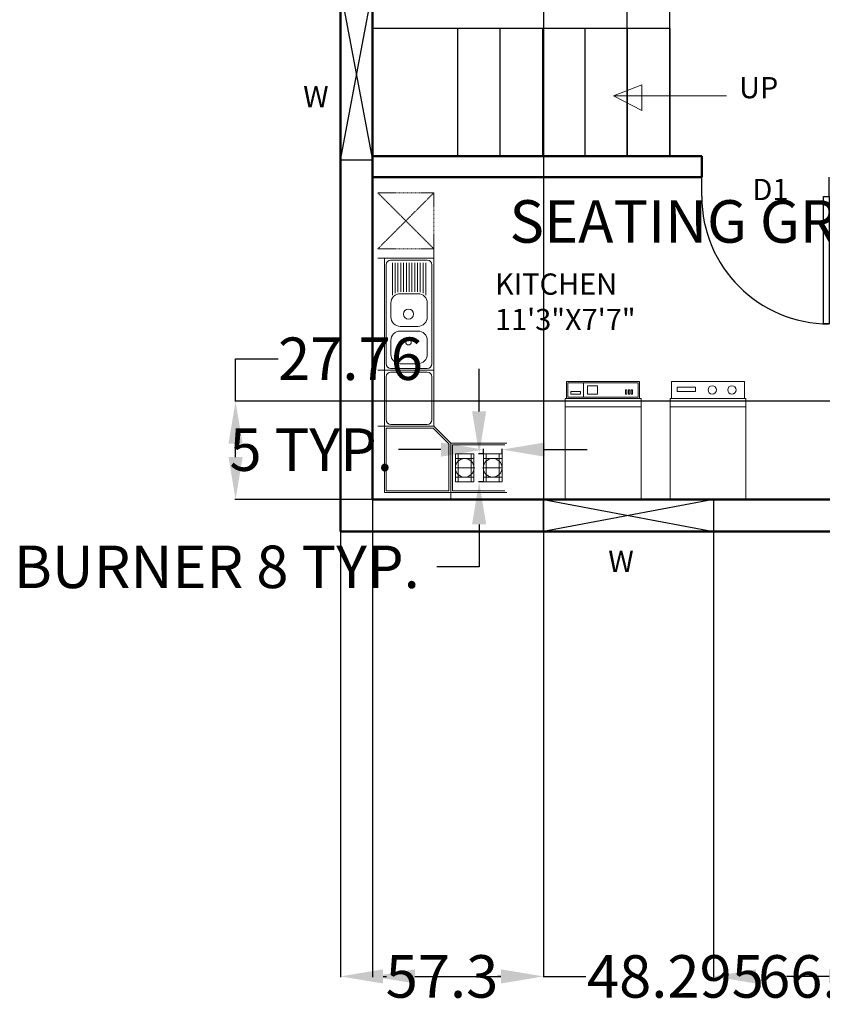
# Model space of a CAD drawing. Units: inches. Extents: x -77 to 516, y -119 to 536.
# Tile 1 of 11: x -77 to 150, y -119 to 159. Entities that reach past the tile are written whole.
import ezdxf

# ---------------------------------------------------------------- set-up
doc = ezdxf.new("R2010")
doc.units = ezdxf.units.IN
doc.header["$MEASUREMENT"] = 0
doc.linetypes.add('HIDDEN', pattern=[0.375, 0.25, -0.125])
for name, color, linetype, lineweight in [('A-ANNO-DIMS', 2, 'Continuous', 18), ('A-ANNO-SYMB', 20, 'Continuous', 18), ('A-AREA-IDEN', 170, 'Continuous', 25), ('A-EQPM', 42, 'Continuous', 18), ('A-FLOR-CASE', 42, 'Continuous', 18), ('A-FLOR-CASE-HIDN', 42, 'HIDDEN', 18), ('A-FLOR-FIXT', 9, 'Continuous', 18), ('A-FLOR-FIXT-PATT', 9, 'Continuous', 13), ('doors', 6, 'Continuous', 25), ('steps', 20, 'Continuous', 25), ('text', 170, 'Continuous', 18), ('walls', 40, 'Continuous', 50), ('windows', 1, 'Continuous', 25)]:
    doc.layers.add(name, color=color, linetype=linetype, lineweight=lineweight)
doc.styles.get("Standard").update_dxf_attribs({"font": 'arial.ttf'})
doc.dimstyles.get("Standard").update_dxf_attribs({"dimtxt": 12, "dimasz": 12, "dimexe": 0.18, "dimexo": 0.0625, "dimgap": 0.09, "dimtad": 0, "dimtih": 1, "dimtoh": 1, "dimdec": 1, "dimzin": 0, "dimdsep": 46, "dimlunit": 4, "dimtxsty": 'Standard', "dimcen": 0.09, "dimadec": 0, "dimazin": 0, "dimtfac": 1, "dimtdec": 1, "dimtofl": 0, "dimtmove": 0, "dimatfit": 3, "dimfxl": 1, "dimtolj": 1, "dimtzin": 0, "dimarcsym": 0})

# ---------------------------------------------------------------- blocks, each defined once
blk = doc.blocks.new('*U2')
for p, q in [((0, 0), (0, -6)), ((40, 0), (40, -6))]:
    blk.add_line(p, q)
blk.add_lwpolyline([(0, 0), (0, 40), (1.75, 40), (1.75, 0)], close=True)
blk.add_arc((0, 0), 40, 0, 90)
blk = doc.blocks.new('WIN-48IN')
for p, q in [((0, 0), (9, 48)), ((0, 48), (9, 0))]:
    blk.add_line(p, q)
blk.add_lwpolyline([(0, 48), (9, 48), (9, 0), (0, 0)], close=True)
blk = doc.blocks.new('COOKTOP-BURNER')
for p, q in [((0, 7.91), (5.27, 7.91)), ((0, 0), (0, 7.91)), ((0, 6.59), (5.27, 6.59)), ((0.79, 0), (0.79, 7.91)), ((4.48, 7.91), (4.48, 0)), ((5.27, 7.91), (5.27, 0)), ((5.27, 3.95), (0, 3.95)), ((5.27, 1.32), (0, 1.32)), ((5.27, 0), (0, 0))]:
    blk.add_line(p, q)
blk.add_circle((2.64, 3.95), 2.64)
blk = doc.blocks.new('*D30')
at = {"layer": 'A-ANNO-DIMS', "color": 0, "lineweight": -2, "transparency": 16777216}
for p, q in [((351.13, 120.17), (351.28, 103.03)), ((237.64, 119.18), (237.79, 102.04)), ((339.28, 103.1), (249.78, 102.32)), ((237.78, 102.22), (225.78, 102.12))]:
    blk.add_line(p, q, dxfattribs=at)
at = {"layer": 'A-ANNO-DIMS', "color": 0, "transparency": 16777216}
for points in [[(249.77, 104.32), (249.8, 100.32), (237.78, 102.22)], [(339.27, 105.1), (339.3, 101.1), (351.28, 103.21)]]:
    blk.add_solid(points, dxfattribs=at)
at = {"layer": 'Defpoints', "color": 0, "transparency": 16777216}
for p in [(351.13, 120.23), (237.64, 119.24), (237.78, 102.22)]:
    blk.add_point(p, dxfattribs=at)
at = {"layer": 'A-ANNO-DIMS', "color": 0, "transparency": 16777216, "insert": (140.3, 102.12), "char_height": 12, "attachment_point": 5}
blk.add_mtext('\\A1;SEATING GROUP 114', dxfattribs=at)
blk = doc.blocks.new('*D34')
at = {"layer": 'A-ANNO-DIMS', "color": 0, "lineweight": -2, "transparency": 16777216}
for p, q in [((52.9, 48.5), (52.9, 60.5)), ((54.02, 36.5), (52.72, 36.5)), ((54.02, 28.59), (52.72, 28.59)), ((52.9, 16.59), (52.9, 4.59)), ((52.9, 4.59), (40.9, 4.59))]:
    blk.add_line(p, q, dxfattribs=at)
at = {"layer": 'A-ANNO-DIMS', "color": 0, "transparency": 16777216}
for points in [[(50.9, 48.5), (54.9, 48.5), (52.9, 36.5)], [(50.9, 16.59), (54.9, 16.59), (52.9, 28.59)]]:
    blk.add_solid(points, dxfattribs=at)
at = {"layer": 'Defpoints', "color": 0, "transparency": 16777216}
for p in [(54.08, 36.5), (52.9, 28.59), (54.08, 28.59)]:
    blk.add_point(p, dxfattribs=at)
at = {"layer": 'A-ANNO-DIMS', "color": 0, "transparency": 16777216, "insert": (-21.2, 4.59), "char_height": 12, "attachment_point": 5}
blk.add_mtext('\\A1;BURNER 8 TYP.', dxfattribs=at)
blk = doc.blocks.new('*D35')
at = {"layer": 'A-ANNO-DIMS', "color": 0, "lineweight": -2, "transparency": 16777216}
for p, q in [((42.08, 37.69), (30.08, 37.69)), ((54.08, 36.57), (54.08, 37.87)), ((59.36, 36.57), (59.36, 37.87)), ((71.36, 37.69), (83.36, 37.69))]:
    blk.add_line(p, q, dxfattribs=at)
at = {"layer": 'A-ANNO-DIMS', "color": 0, "transparency": 16777216}
for points in [[(42.08, 39.69), (42.08, 35.69), (54.08, 37.69)], [(71.36, 39.69), (71.36, 35.69), (59.36, 37.69)]]:
    blk.add_solid(points, dxfattribs=at)
at = {"layer": 'Defpoints', "color": 0, "transparency": 16777216}
for p in [(54.08, 37.69), (54.08, 36.5), (59.36, 36.5)]:
    blk.add_point(p, dxfattribs=at)
at = {"layer": 'A-ANNO-DIMS', "color": 0, "transparency": 16777216, "insert": (5.45, 37.69), "char_height": 12, "attachment_point": 5}
blk.add_mtext('\\A1;5 TYP.', dxfattribs=at)
blk = doc.blocks.new('*D39')
at = {"layer": 'A-ANNO-DIMS', "color": 0, "lineweight": -2, "transparency": 16777216}
for p, q in [((22.75, 485.53), (22.75, -111.24)), ((71.05, 485.53), (71.05, -111.24)), ((34.75, -111.06), (59.05, -111.06)), ((71.05, -111.06), (83.05, -111.06))]:
    blk.add_line(p, q, dxfattribs=at)
at = {"layer": 'A-ANNO-DIMS', "color": 0, "transparency": 16777216}
for points in [[(34.75, -109.06), (34.75, -113.06), (22.75, -111.06)], [(59.05, -109.06), (59.05, -113.06), (71.05, -111.06)]]:
    blk.add_solid(points, dxfattribs=at)
at = {"layer": 'Defpoints', "color": 0, "transparency": 16777216}
for p in [(22.75, 485.59), (71.05, 485.59), (71.05, -111.06)]:
    blk.add_point(p, dxfattribs=at)
at = {"layer": 'A-ANNO-DIMS', "color": 0, "transparency": 16777216, "insert": (108.33, -111.06), "char_height": 12, "attachment_point": 5}
blk.add_mtext('\\A1;48.295', dxfattribs=at)
blk = doc.blocks.new('*D40')
at = {"layer": 'A-ANNO-DIMS', "color": 0, "lineweight": -2, "transparency": 16777216}
for p, q in [((163.750061, 485.5259), (163.750061, -111.2416)), ((184.750061, 485.5259), (184.750061, -111.2416)), ((151.750061, -111.0616), (139.750061, -111.0616)), ((196.750061, -111.0616), (208.750061, -111.0616))]:
    blk.add_line(p, q, dxfattribs=at)
at = {"layer": 'A-ANNO-DIMS', "color": 0, "transparency": 16777216}
for points in [[(151.750061, -109.0616), (151.750061, -113.0616), (163.750061, -111.0616)], [(196.750061, -109.0616), (196.750061, -113.0616), (184.750061, -111.0616)]]:
    blk.add_solid(points, dxfattribs=at)
at = {"layer": 'Defpoints', "color": 0, "transparency": 16777216}
for p in [(163.750061, 485.5884), (184.750061, 485.5884), (184.750061, -111.0616)]:
    blk.add_point(p, dxfattribs=at)
at = {"layer": 'A-ANNO-DIMS', "color": 0, "transparency": 16777216, "insert": (174.250061, -111.0616), "char_height": 12, "attachment_point": 5}
blk.add_mtext('\\A1;21', dxfattribs=at)
blk = doc.blocks.new('*D45')
at = {"layer": 'A-ANNO-DIMS', "color": 0, "lineweight": -2, "transparency": 16777216}
for p, q in [((-15.9, 51.35), (-15.9, 63.35)), ((-15.9, 63.35), (-3.9, 63.35)), ((364.69, 51.35), (-16.08, 51.35)), ((-15.9, 35.59), (-15.9, 39.35)), ((364.69, 23.59), (-16.08, 23.59))]:
    blk.add_line(p, q, dxfattribs=at)
at = {"layer": 'A-ANNO-DIMS', "color": 0, "transparency": 16777216}
for points in [[(-17.9, 39.35), (-13.9, 39.35), (-15.9, 51.35)], [(-17.9, 35.59), (-13.9, 35.59), (-15.9, 23.59)]]:
    blk.add_solid(points, dxfattribs=at)
at = {"layer": 'Defpoints', "color": 0, "transparency": 16777216}
for p in [(-15.9, 51.35), (364.75, 51.35), (364.75, 23.59)]:
    blk.add_point(p, dxfattribs=at)
at = {"layer": 'A-ANNO-DIMS', "color": 0, "transparency": 16777216, "insert": (16.54, 63.35), "char_height": 12, "attachment_point": 5}
blk.add_mtext('\\A1;27.76', dxfattribs=at)
blk = doc.blocks.new('*D49')
at = {"layer": 'A-ANNO-DIMS', "color": 0, "lineweight": -2, "transparency": 16777216}
for p, q in [((13.75, 14.53), (13.75, -111.24)), ((71.05, 14.53), (71.05, -111.24)), ((25.75, -111.06), (26.72, -111.06)), ((59.05, -111.06), (58.07, -111.06))]:
    blk.add_line(p, q, dxfattribs=at)
at = {"layer": 'A-ANNO-DIMS', "color": 0, "transparency": 16777216}
for points in [[(25.75, -109.06), (25.75, -113.06), (13.75, -111.06)], [(59.05, -109.06), (59.05, -113.06), (71.05, -111.06)]]:
    blk.add_solid(points, dxfattribs=at)
at = {"layer": 'Defpoints', "color": 0, "transparency": 16777216}
for p in [(13.75, 14.59), (71.05, 14.59), (71.05, -111.06)]:
    blk.add_point(p, dxfattribs=at)
at = {"layer": 'A-ANNO-DIMS', "color": 0, "transparency": 16777216, "insert": (42.4, -111.06), "char_height": 12, "attachment_point": 5}
blk.add_mtext('\\A1;57.3', dxfattribs=at)
blk = doc.blocks.new('*D50')
at = {"layer": 'A-ANNO-DIMS', "color": 0, "lineweight": -2, "transparency": 16777216}
for p, q in [((119.05, 14.53), (119.05, -111.24)), ((185.2, 14.53), (185.2, -111.24)), ((131.05, -111.06), (131.76, -111.06)), ((173.2, -111.06), (172.49, -111.06))]:
    blk.add_line(p, q, dxfattribs=at)
at = {"layer": 'A-ANNO-DIMS', "color": 0, "transparency": 16777216}
for points in [[(131.05, -109.06), (131.05, -113.06), (119.05, -111.06)], [(173.2, -109.06), (173.2, -113.06), (185.2, -111.06)]]:
    blk.add_solid(points, dxfattribs=at)
at = {"layer": 'Defpoints', "color": 0, "transparency": 16777216}
for p in [(119.05, 14.59), (185.2, 14.59), (185.2, -111.06)]:
    blk.add_point(p, dxfattribs=at)
at = {"layer": 'A-ANNO-DIMS', "color": 0, "transparency": 16777216, "insert": (152.12, -111.06), "char_height": 12, "attachment_point": 5}
blk.add_mtext('\\A1;66.16', dxfattribs=at)
blk = doc.blocks.new('*D54')
at = {"layer": 'A-ANNO-DIMS', "color": 0, "lineweight": -2, "transparency": 16777216}
for p, q in [((82.75, 524.95), (70.75, 524.95)), ((94.75, 120.65), (94.75, 525.13)), ((106.75, 120.65), (106.75, 525.13)), ((118.75, 524.95), (130.75, 524.95))]:
    blk.add_line(p, q, dxfattribs=at)
at = {"layer": 'A-ANNO-DIMS', "color": 0, "transparency": 16777216}
for points in [[(82.75, 526.95), (82.75, 522.95), (94.75, 524.95)], [(118.75, 526.95), (118.75, 522.95), (106.75, 524.95)]]:
    blk.add_solid(points, dxfattribs=at)
at = {"layer": 'Defpoints', "color": 0, "transparency": 16777216}
for p in [(106.75, 524.95), (94.75, 120.59), (106.75, 120.59)]:
    blk.add_point(p, dxfattribs=at)
at = {"layer": 'A-ANNO-DIMS', "color": 0, "transparency": 16777216, "insert": (138.81, 524.95), "char_height": 12, "attachment_point": 5}
blk.add_mtext('\\A1;12', dxfattribs=at)

msp = doc.modelspace()

# ---------------------------------------------------------------- hatches: boundary and pattern name
at = {"layer": 'A-FLOR-FIXT-PATT'}
h = msp.add_hatch(dxfattribs=at)
h.set_pattern_fill('ANSI31', color=256, scale=6.3086, angle=45, style=0)
h.paths.add_polyline_path([(28.3742, 81.3195), (29.1652, 81.8982), (29.9563, 82.1807), (30.7473, 82.2501), (31.5383, 82.2501), (32.3293, 82.2501), (33.1203, 82.2501), (33.9114, 82.2501), (34.7024, 82.2501), (35.4934, 82.2501), (36.2844, 82.1807), (37.0754, 81.8982), (37.8665, 81.3195), (37.8665, 90.424), (28.3742, 90.424)])

# ---------------------------------------------------------------- linework, layer by layer
at = {"layer": 'A-ANNO-SYMB'}
for p, q in [((90.8387, 137.5471), (98.8706, 140.7268)), ((98.8706, 140.7268), (98.8706, 133.4676)), ((122.7454, 137.5471), (90.8387, 137.5471)), ((98.8706, 133.4676), (90.8387, 137.5471))]:
    msp.add_line(p, q, dxfattribs=at)
at = {"layer": 'A-EQPM'}
for p, q in [((77.5865, 56.9118), (98.2153, 56.9118)), ((77.5865, 56.9118), (77.5865, 52.1513)), ((77.9832, 56.5151), (97.8186, 56.5151)), ((77.9832, 52.5481), (77.9832, 56.5151)), ((82.347, 52.5481), (82.347, 56.5151)), ((83.5371, 53.3415), (83.5371, 55.7217)), ((83.5371, 55.7217), (86.3141, 55.7217)), ((86.3141, 55.7217), (86.3141, 53.3415)), ((97.8186, 56.5151), (97.8186, 52.5481)), ((98.2153, 56.9118), (98.2153, 52.1513)), ((107.2246, 56.9118), (127.8534, 56.9118)), ((107.2246, 56.9118), (107.2246, 52.1513)), ((127.8534, 56.9118), (127.8534, 52.1513)), ((81.5536, 54.1349), (78.7767, 54.1349)), ((78.7767, 54.1349), (78.7767, 53.3415)), ((78.7767, 53.3415), (81.5536, 53.3415)), ((81.5536, 53.3415), (81.5536, 54.1349)), ((86.3141, 53.3415), (83.5371, 53.3415)), ((94.2483, 53.3415), (94.2483, 54.5316)), ((94.2483, 54.5316), (94.645, 54.5316)), ((94.645, 53.3415), (94.2483, 53.3415)), ((94.645, 54.5316), (94.645, 53.3415)), ((95.0417, 53.3415), (95.0417, 54.5316)), ((95.0417, 54.5316), (95.4384, 54.5316)), ((95.4384, 53.3415), (95.0417, 53.3415)), ((95.4384, 54.5316), (95.4384, 53.3415)), ((95.8351, 53.3415), (95.8351, 54.5316)), ((95.8351, 54.5316), (96.2318, 54.5316)), ((96.2318, 53.3415), (95.8351, 53.3415)), ((96.2318, 54.5316), (96.2318, 53.3415)), ((108.8114, 55.325), (113.9686, 55.325)), ((108.8114, 54.1349), (108.8114, 55.325)), ((113.9686, 54.1349), (108.8114, 54.1349)), ((113.9686, 55.325), (113.9686, 54.1349)), ((77.1898, 23.5884), (77.1898, 52.1513)), ((77.1898, 52.1513), (98.612, 52.1513)), ((97.8186, 52.5481), (77.9832, 52.5481)), ((98.612, 52.1513), (98.612, 23.5884)), ((106.8279, 52.1513), (128.2501, 52.1513)), ((106.8279, 23.5884), (106.8279, 52.1513)), ((128.2501, 52.1513), (128.2501, 23.5884)), ((77.1898, 49.7711), (98.612, 49.7711)), ((106.8279, 49.7711), (128.2501, 49.7711)), ((60.6742, 39.535), (44.8538, 39.535)), ((45.3811, 39.0077), (45.3811, 26.0877)), ((60.1468, 39.0077), (45.3811, 39.0077)), ((44.8538, 25.5603), (60.6742, 25.5603)), ((45.3811, 26.0877), (60.1468, 26.0877)), ((77.1898, 23.5884), (98.612, 23.5884)), ((106.8279, 23.5884), (128.2501, 23.5884))]:
    msp.add_line(p, q, dxfattribs=at)
for centre in [(118.7291, 54.5316), (124.283, 54.5316)]:
    msp.add_circle(centre, 1.1901, dxfattribs=at)
at = {"layer": 'A-FLOR-CASE'}
for p, q in [((40.1077, 60.1015), (40.1077, 94.3791)), ((24.2873, 91.7423), (40.1077, 91.7423)), ((26.133, 91.7423), (26.133, 60.1015)), ((40.1077, 60.1015), (24.2873, 60.1015)), ((26.133, 60.1015), (26.133, 44.2811)), ((38.262, 59.5742), (27.9787, 59.5742)), ((40.1077, 44.2811), (40.1077, 60.1015)), ((26.6603, 58.2558), (26.6603, 46.1268)), ((39.5803, 46.1268), (39.5803, 58.2558)), ((27.9787, 44.8085), (38.262, 44.8085)), ((24.2873, 44.2811), (40.1077, 44.2811)), ((26.133, 25.5603), (26.133, 44.2811)), ((26.6603, 43.7538), (39.8892, 43.7538)), ((26.6603, 26.0877), (26.6603, 43.7538)), ((39.8892, 43.7538), (44.3265, 39.3166)), ((40.1077, 44.2811), (44.8538, 39.535)), ((44.3265, 39.3166), (44.3265, 26.0877)), ((44.8538, 39.535), (44.8538, 23.7146)), ((44.8538, 25.5603), (26.133, 25.5603)), ((44.3265, 26.0877), (26.6603, 26.0877))]:
    msp.add_line(p, q, dxfattribs=at)
for centre, start, end in [((27.9787, 58.2558), 90, 180), ((38.262, 58.2558), 0, 90), ((27.9787, 46.1268), 180, 270), ((38.262, 46.1268), 270, 0)]:
    msp.add_arc(centre, 1.3184, start, end, dxfattribs=at)
at = {"layer": 'A-FLOR-CASE-HIDN'}
for p, q in [((24.2873, 110.1994), (40.1077, 110.1994)), ((24.2873, 94.3791), (40.1077, 110.1994)), ((24.2873, 110.1994), (40.1077, 94.3791)), ((40.1077, 110.1994), (40.1077, 94.3791)), ((24.2873, 94.3791), (40.1077, 94.3791))]:
    msp.add_line(p, q, dxfattribs=at)
at = {"layer": 'A-FLOR-FIXT'}
for p, q in [((26.6603, 89.8966), (26.6603, 61.9472)), ((38.262, 91.215), (27.9787, 91.215)), ((39.5803, 61.9472), (39.5803, 89.8966)), ((30.6154, 81.7227), (35.6252, 81.7227)), ((27.9787, 79.086), (27.9787, 75.1309)), ((38.262, 75.1309), (38.262, 79.086)), ((30.6154, 72.4942), (35.6252, 72.4942)), ((30.6154, 71.1758), (35.6252, 71.1758)), ((27.9787, 68.5391), (27.9787, 64.584)), ((38.262, 64.584), (38.262, 68.5391)), ((30.6154, 61.9472), (35.6252, 61.9472)), ((27.9787, 60.6289), (38.262, 60.6289))]:
    msp.add_line(p, q, dxfattribs=at)
for centre, radius in [((32.9438, 75.9512), 1.4037), ((32.9438, 68.044), 0.7986)]:
    msp.add_circle(centre, radius, dxfattribs=at)
for centre, radius, start, end in [((27.9787, 89.8966), 1.3184, 90, 180), ((38.262, 89.8966), 1.3184, 0, 90), ((30.6154, 79.086), 2.6367, 90, 180), ((35.6252, 79.086), 2.6367, 0, 90), ((30.6154, 75.1309), 2.6367, 180, 270), ((35.6252, 75.1309), 2.6367, 270, 0), ((30.6154, 68.5391), 2.6367, 90, 180), ((35.6252, 68.5391), 2.6367, 0, 90), ((30.6154, 64.584), 2.6367, 180, 270), ((35.6252, 64.584), 2.6367, 270, 0), ((27.9787, 61.9472), 1.3184, 180, 270), ((38.262, 61.9472), 1.3184, 270, 0)]:
    msp.add_arc(centre, radius, start, end, dxfattribs=at)
at = {"layer": 'steps'}
for p, q in [((106.7501, 156.5884), (22.7501, 156.5884)), ((46.7501, 156.5884), (46.7501, 120.5884)), ((58.7501, 156.5884), (58.7501, 120.5884)), ((70.7501, 156.5884), (70.7501, 120.5884)), ((82.7501, 156.5884), (82.7501, 120.5884)), ((94.7501, 156.5884), (94.7501, 120.5884)), ((106.7501, 156.5884), (106.7501, 120.5884))]:
    msp.add_line(p, q, dxfattribs=at)
at = {"layer": 'walls'}
for p, q in [((22.7501, 335.5884), (22.7501, 23.5884)), ((22.7501, 120.5884), (115.7501, 120.5884)), ((115.7501, 120.5884), (115.7501, 114.5884)), ((22.7501, 114.5884), (115.7501, 114.5884)), ((22.7501, 23.5884), (233.7501, 23.5884))]:
    msp.add_line(p, q, dxfattribs=at)
msp.add_lwpolyline([(373.7501, 131.5884), (373.7501, 494.5884), (13.7501, 494.5884), (13.7501, 14.5884), (239.7501, 14.5884)], dxfattribs=at)

# ---------------------------------------------------------------- block references
at = {"layer": 'A-EQPM'}
msp.add_blockref('COOKTOP-BURNER', (46.172, 28.593), dxfattribs=at)
at = {"layer": 'A-EQPM', "rotation": 180}
msp.add_blockref('COOKTOP-BURNER', (59.356, 36.5023), dxfattribs=at)
at = {"layer": 'doors', "xscale": 0.9000000000000007, "yscale": 0.9000000000000007, "zscale": 0.9000000000000007, "rotation": 180}
msp.add_blockref('*U2', (151.7501, 109.1884), dxfattribs=at)
at = {"layer": 'windows'}
msp.add_blockref('WIN-48IN', (13.75, 119.4084), dxfattribs=at)
at = {"layer": 'windows', "rotation": 270}
msp.add_blockref('WIN-48IN', (71.0456, 23.5885), dxfattribs=at)

# ---------------------------------------------------------------- texts
at = {"layer": 'A-AREA-IDEN', "insert": (57.3651, 87.4281), "char_height": 6, "attachment_point": 1}
msp.add_mtext_dynamic_manual_height_columns('KITCHEN\\P11\'3"X7\'7"', width=105.041962, gutter_width=1, heights=[0], dxfattribs=at)
at = {"layer": 'text', "char_height": 6, "attachment_point": 1}
for s, insert in [('UP', (126.3082, 142.9061)), ('W', (3.1967, 140.3738)), ('D1', (130.0832, 114.1322)), ('W', (89.371, 9.1157))]:
    msp.add_mtext_dynamic_manual_height_columns(s, width=105.041962, gutter_width=1, heights=[0], dxfattribs=dict(at, insert=insert))

# ---------------------------------------------------------------- dimensions: what is measured, and where the dimension line sits
at = {"layer": 'A-ANNO-DIMS'}
for base, p1, p2, override, picture, middle in [((106.7501, 524.9457), (94.7501, 120.5884), (106.7501, 120.5884), {"dimdec": 0, "dimlfac": 1, "dimrnd": 0, "dimzin": 0, "dimdsep": 46, "dimlunit": 2}, '*D54', (138.8087, 524.9457)), ((71.0451, -111.0616), (22.7501, 485.5884), (71.0451, 485.5884), {"dimdec": 3, "dimlfac": 1, "dimrnd": 0, "dimzin": 0, "dimdsep": 46, "dimlunit": 2}, '*D39', (108.3302, -111.0616)), ((184.7501, -111.0616), (163.7501, 485.5884), (184.7501, 485.5884), {"dimdec": 0, "dimlfac": 1, "dimrnd": 0, "dimzin": 0, "dimdsep": 46, "dimlunit": 2}, '*D40', (174.2501, -111.0616)), ((71.0451, -111.0616), (13.7501, 14.5884), (71.0451, 14.5884), {"dimdec": 1, "dimlfac": 1, "dimrnd": 0, "dimzin": 0, "dimdsep": 46, "dimlunit": 2}, '*D49', (42.3976, -111.0616)), ((185.2037, -111.0616), (119.0451, 14.5884), (185.2037, 14.5884), {"dimdec": 2, "dimlfac": 1, "dimrnd": 0, "dimzin": 0, "dimdsep": 46, "dimlunit": 2}, '*D50', (152.1244, -111.0616))]:
    dim = msp.add_linear_dim(base=base, p1=p1, p2=p2, dimstyle='Standard', override=override, dxfattribs=at)
    dim.commit()
    dim.dimension.update_dxf_attribs({"geometry": picture, "text_midpoint": middle})
for base, p1, p2, angle, text, picture, middle in [((237.7836, 102.22), (351.1342, 120.231), (237.6357, 119.2448), 180.497807, 'SEATING GROUP <>', '*D30', (140.3025, 102.1158)), ((52.8958, 28.5926), (54.0824, 36.5028), (54.0824, 28.5926), 270, 'BURNER <> TYP.', '*D34', (-21.1955, 4.5926)), ((54.0824, 37.6893), (59.3558, 36.5028), (54.0824, 36.5028), 180, '<> TYP.', '*D35', (5.448, 37.6893))]:
    dim = msp.add_linear_dim(base=base, p1=p1, p2=p2, angle=angle, text=text, dimstyle='Standard', override={"dimdec": 0, "dimlfac": 1, "dimrnd": 0, "dimzin": 0, "dimdsep": 46, "dimlunit": 2}, dxfattribs=at)
    dim.commit()
    dim.dimension.update_dxf_attribs({"geometry": picture, "text_midpoint": middle})
dim = msp.add_linear_dim(base=(-15.8999, 51.3473), p1=(364.7501, 23.5884), p2=(364.7501, 51.3473), angle=90, dimstyle='Standard', override={"dimdec": 2, "dimlfac": 1, "dimrnd": 0, "dimzin": 0, "dimdsep": 46, "dimlunit": 2}, dxfattribs=at)
dim.commit()
dim.dimension.update_dxf_attribs({"geometry": '*D45', "text_midpoint": (16.5352, 63.3473)})

doc.saveas('drawing.dxf')
